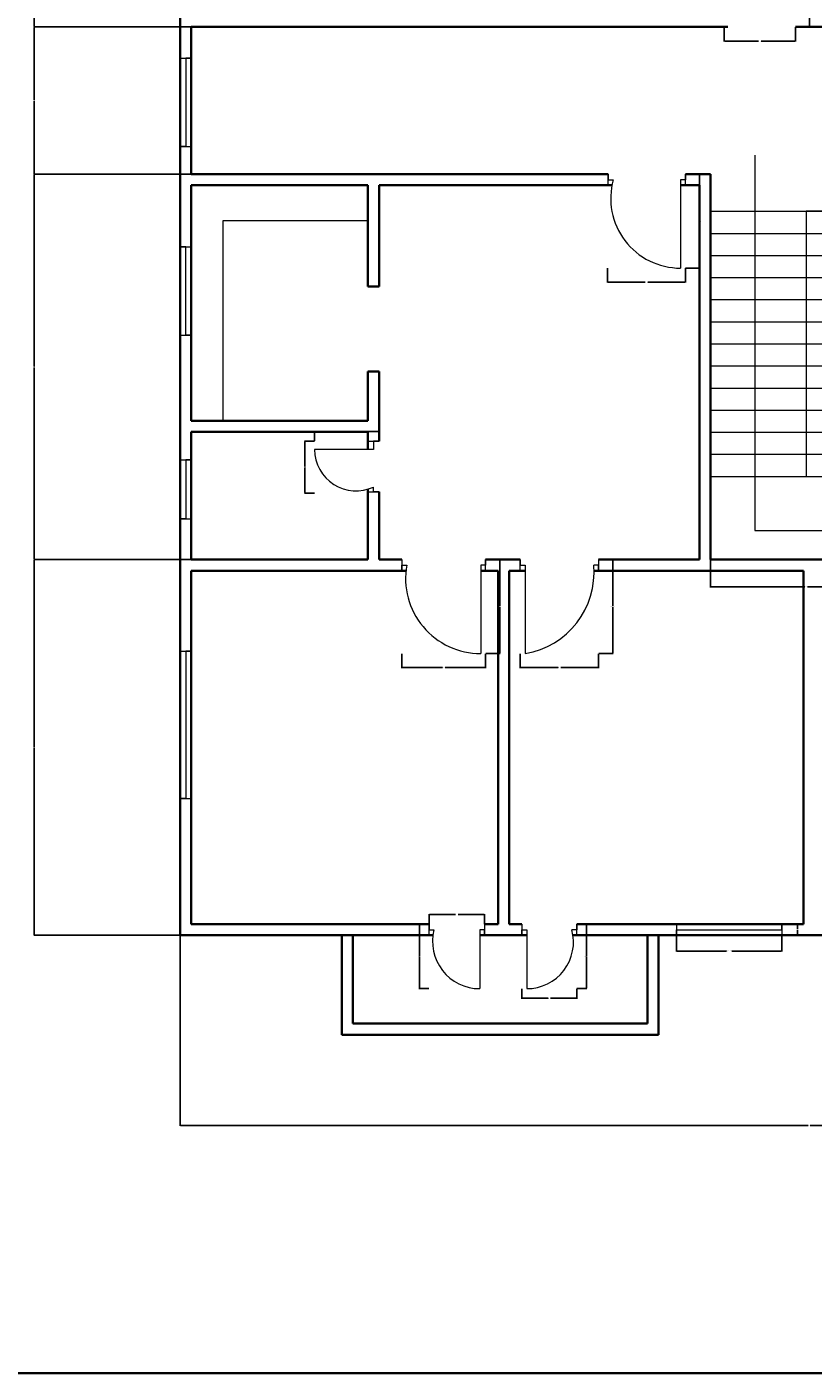
# Model space of a CAD drawing. Units: inches. Extents: x 1944 to 3454, y 1352 to 3055.
# Tile 10 of 17: x 2582 to 2903, y 1352 to 1900. Entities that reach past the tile are written whole.
import ezdxf

# ---------------------------------------------------------------- set-up
doc = ezdxf.new("R2010")
doc.units = ezdxf.units.IN
for name, color, linetype, lineweight in [('A-ANNO-DIMS', 2, 'Continuous', 18), ('A-ANNO-TTLB', 7, 'Continuous', 35), ('A-DOOR', 3, 'Continuous', 20), ('A-FLOR-CASE', 8, 'Continuous', 20), ('A-FLOR-STRS', 7, 'Continuous', 20), ('A-GLAZ', 4, 'Continuous', 18), ('A-WALL', 7, 'Continuous', 35)]:
    doc.layers.add(name, color=color, linetype=linetype, lineweight=lineweight)
doc.styles.get("Standard").update_dxf_attribs({"font": 'arial.ttf'})
doc.dimstyles.get("Standard").update_dxf_attribs({"dimtxt": 0.18, "dimasz": 0.18, "dimexe": 0.18, "dimexo": 0.0625, "dimgap": 0.09, "dimtad": 0, "dimtih": 1, "dimtoh": 1, "dimdec": 4, "dimzin": 0, "dimdsep": 46, "dimtxsty": 'Standard', "dimcen": 0.09, "dimadec": 0, "dimazin": 0, "dimtfac": 1, "dimtdec": 4, "dimtofl": 0, "dimtmove": 0, "dimatfit": 3, "dimfxl": 1, "dimtolj": 1, "dimtzin": 0, "dimarcsym": 0})

# ---------------------------------------------------------------- blocks, each defined once
blk = doc.blocks.new('DOOR-SWING-24IN-08')
for p, q in [((24, 17.34), (0, 17.34)), ((21.75, 20.75), (26.25, 20.75)), ((26.25, 20.75), (24, 20.75)), ((24, 20.75), (24, 19.34)), ((24, 19.34), (24, 17.34)), ((21.75, 0), (26.25, 0)), ((24, 0), (24, 2)), ((26.25, 0), (24, 0))]:
    blk.add_line(p, q)
blk.add_arc((16.9, 17.34), 16.9, 180, 294.8206)
blk = doc.blocks.new('DOOR-SWING-36IN-07')
for p, q in [((0, 38.25), (0, 33.75)), ((0, 33.75), (0, 36)), ((0, 36), (2, 36)), ((34.17, 36), (32.17, 36)), ((32.17, 36), (32.17, 0)), ((34.17, 33.75), (34.17, 38.25)), ((34.17, 38.25), (34.17, 36))]:
    blk.add_line(p, q)
blk.add_arc((32.17, 30.64), 30.64, 169.9223, 270)
blk = doc.blocks.new('DOOR-SWING-36IN-08')
for p, q in [((0, 33.75), (0, 38.25)), ((0, 38.25), (0, 38.25)), ((0, 38.25), (0, 36)), ((0, 36), (2, 36)), ((2, 36), (2, 0)), ((31.9, 36), (29.9, 36)), ((31.9, 38.25), (31.9, 33.75)), ((31.9, 33.75), (31.9, 36))]:
    blk.add_line(p, q)
blk.add_arc((-3.46, 33.05), 33.5, 279.3869, 5.0549)
blk = doc.blocks.new('DOOR-SWING-24IN-09')
for p, q in [((0, 21.75), (0, 26.25)), ((0, 26.25), (0, 24)), ((0, 24), (2, 24)), ((22.65, 24), (20.65, 24)), ((20.65, 24), (20.65, 0)), ((22.65, 26.25), (22.65, 21.75)), ((22.65, 21.75), (22.65, 24)), ((22.65, 21.75), (22.65, 21.75))]:
    blk.add_line(p, q)
blk.add_arc((20.65, 19.25), 19.25, 165.7058, 270)
blk = doc.blocks.new('DOOR-SWING-24IN-10')
for p, q in [((0, 26.25), (0, 21.75)), ((0, 21.75), (0, 24)), ((0, 24), (2, 24)), ((2, 24), (2, 0)), ((22.35, 24), (20.35, 24)), ((22.35, 21.75), (22.35, 26.25)), ((22.35, 26.25), (22.35, 24))]:
    blk.add_line(p, q)
blk.add_arc((2, 19.01), 19.01, 270, 15.2011)
blk = doc.blocks.new('DOOR-SWING-36IN-11')
for p, q in [((0, 33.75), (0, 38.25)), ((0, 38.25), (0, 36)), ((0, 36), (2, 36)), ((31.41, 36), (29.41, 36)), ((29.41, 36), (29.41, 0)), ((31.41, 33.75), (31.41, 38.25)), ((31.41, 38.25), (31.41, 36))]:
    blk.add_line(p, q)
blk.add_arc((29.41, 28.43), 28.43, 164.5673, 270)
blk = doc.blocks.new('WINDOW-PLAN-60.00IN-02')
for p, q in [((2.25, 60), (0, 60)), ((0, 60), (4.5, 60)), ((2.25, 0), (2.25, 60)), ((0, 0), (4.5, 0)), ((4.5, 0), (2.25, 0))]:
    blk.add_line(p, q)
blk = doc.blocks.new('WINDOW-PLAN-36.00IN-01')
for p, q in [((0, 36), (4.5, 36)), ((4.5, 36), (2.25, 36)), ((2.25, 36), (2.25, 0)), ((2.25, 0), (0, 0)), ((0, 0), (4.5, 0))]:
    blk.add_line(p, q)
blk = doc.blocks.new('WINDOW-PLAN-24.00IN-01')
for p, q in [((2.25, 24), (0, 24)), ((0, 24), (4.5, 24)), ((2.25, 0), (2.25, 24)), ((0, 0), (4.5, 0)), ((4.5, 0), (2.25, 0))]:
    blk.add_line(p, q)
blk = doc.blocks.new('WINDOW-PLAN-42.86IN-01')
for p, q in [((0, 4.5), (0, 0)), ((0, 0), (0, 2.25)), ((0, 2.25), (42.86, 2.25)), ((42.86, 2.25), (42.86, 4.5)), ((42.86, 4.5), (42.86, 0))]:
    blk.add_line(p, q)
blk = doc.blocks.new('STAIR-TWO-FLIGHT-01')
for p, q in [((18.12, 152.99), (18.12, 0)), ((0, 130.08), (78, 130.08)), ((78, 130.08), (39, 130.08)), ((39, 130.08), (39, 22.08)), ((0, 121.08), (78, 121.08)), ((0, 112.08), (78, 112.08)), ((0, 103.08), (78, 103.08)), ((0, 94.08), (78, 94.08)), ((0, 85.08), (78, 85.08)), ((0, 76.08), (78, 76.08)), ((0, 67.08), (78, 67.08)), ((61.93, 0), (61.93, 67.08)), ((0, 58.08), (78, 58.08)), ((0, 49.08), (78, 49.08)), ((0, 40.08), (78, 40.08)), ((0, 31.08), (78, 31.08)), ((0, 22.08), (78, 22.08)), ((18.12, 0), (61.93, 0))]:
    blk.add_line(p, q)
blk = doc.blocks.new('*D84')
at = {"layer": 'A-ANNO-DIMS', "color": 0, "lineweight": -2, "transparency": 16777216}
for p, q in [((2847.08, 1530.03), (2847.08, 1523.49)), ((2889.94, 1530.03), (2889.94, 1523.49)), ((2847.26, 1523.67), (2867.39, 1523.67)), ((2889.76, 1523.67), (2869.63, 1523.67))]:
    blk.add_line(p, q, dxfattribs=at)
at = {"layer": 'A-ANNO-DIMS', "color": 0, "transparency": 16777216}
for points in [[(2847.26, 1523.7), (2847.26, 1523.64), (2847.08, 1523.67)], [(2889.76, 1523.7), (2889.76, 1523.64), (2889.94, 1523.67)]]:
    blk.add_solid(points, dxfattribs=at)
at = {"layer": 'Defpoints', "color": 0, "transparency": 16777216}
for p in [(2847.08, 1530.1), (2889.94, 1530.1), (2889.94, 1523.67)]:
    blk.add_point(p, dxfattribs=at)
at = {"layer": 'A-ANNO-DIMS', "color": 0, "transparency": 16777216, "insert": (2868.51, 1523.67), "char_height": 0.18, "attachment_point": 5}
blk.add_mtext('\\A1;WINDOW 43 TYP.', dxfattribs=at)
blk = doc.blocks.new('*D85')
at = {"layer": 'A-ANNO-DIMS', "color": 0, "lineweight": -2, "transparency": 16777216}
for p, q in [((2890, 1534.6), (2896.55, 1534.6)), ((2890, 1530.1), (2896.55, 1530.1)), ((2896.37, 1534.42), (2896.37, 1532.53)), ((2896.37, 1530.28), (2896.37, 1532.16))]:
    blk.add_line(p, q, dxfattribs=at)
at = {"layer": 'A-ANNO-DIMS', "color": 0, "transparency": 16777216}
for points in [[(2896.34, 1534.42), (2896.4, 1534.42), (2896.37, 1534.6)], [(2896.34, 1530.28), (2896.4, 1530.28), (2896.37, 1530.1)]]:
    blk.add_solid(points, dxfattribs=at)
at = {"layer": 'Defpoints', "color": 0, "transparency": 16777216}
for p in [(2889.94, 1534.6), (2889.94, 1530.1), (2896.37, 1534.6)]:
    blk.add_point(p, dxfattribs=at)
at = {"layer": 'A-ANNO-DIMS', "color": 0, "transparency": 16777216, "insert": (2896.37, 1532.35), "char_height": 0.18, "attachment_point": 5}
blk.add_mtext('\\A1;5 TYP.', dxfattribs=at)
blk = doc.blocks.new('*D91')
at = {"layer": 'A-ANNO-DIMS', "color": 0, "lineweight": -2, "transparency": 16777216}
for p, q in [((2860.88, 1694.86), (2860.88, 1671.8)), ((2938.88, 1694.86), (2938.88, 1671.8)), ((2861.06, 1671.98), (2899.35, 1671.98)), ((2938.7, 1671.98), (2900.4, 1671.98))]:
    blk.add_line(p, q, dxfattribs=at)
at = {"layer": 'A-ANNO-DIMS', "color": 0, "transparency": 16777216}
for points in [[(2861.06, 1672.01), (2861.06, 1671.95), (2860.88, 1671.98)], [(2938.7, 1672.01), (2938.7, 1671.95), (2938.88, 1671.98)]]:
    blk.add_solid(points, dxfattribs=at)
at = {"layer": 'Defpoints', "color": 0, "transparency": 16777216}
for p in [(2860.88, 1694.92), (2938.88, 1694.92), (2938.88, 1671.98)]:
    blk.add_point(p, dxfattribs=at)
at = {"layer": 'A-ANNO-DIMS', "color": 0, "transparency": 16777216, "insert": (2899.88, 1671.98), "char_height": 0.18, "attachment_point": 5}
blk.add_mtext('\\A1;78 TYP.', dxfattribs=at)
blk = doc.blocks.new('*D104')
at = {"layer": 'A-ANNO-DIMS', "color": 0, "lineweight": -2, "transparency": 16777216}
for p, q in [((2769.38, 1683.1), (2775.23, 1683.1)), ((2775.05, 1682.92), (2775.05, 1664.15)), ((2775.05, 1645.03), (2775.05, 1663.79)), ((2769.38, 1644.85), (2775.23, 1644.85))]:
    blk.add_line(p, q, dxfattribs=at)
at = {"layer": 'A-ANNO-DIMS', "color": 0, "transparency": 16777216}
for points in [[(2775.02, 1682.92), (2775.08, 1682.92), (2775.05, 1683.1)], [(2775.02, 1645.03), (2775.08, 1645.03), (2775.05, 1644.85)]]:
    blk.add_solid(points, dxfattribs=at)
at = {"layer": 'Defpoints', "color": 0, "transparency": 16777216}
for p in [(2769.32, 1683.1), (2775.05, 1683.1), (2769.32, 1644.85)]:
    blk.add_point(p, dxfattribs=at)
at = {"layer": 'A-ANNO-DIMS', "color": 0, "transparency": 16777216, "insert": (2775.05, 1663.97), "char_height": 0.18, "attachment_point": 5}
blk.add_mtext('\\A1;SWING 38 TYP.', dxfattribs=at)
blk = doc.blocks.new('*D105')
at = {"layer": 'A-ANNO-DIMS', "color": 0, "lineweight": -2, "transparency": 16777216}
for p, q in [((2735.15, 1644.78), (2735.15, 1638.93)), ((2769.32, 1644.78), (2769.32, 1638.93)), ((2735.33, 1639.11), (2751.71, 1639.11)), ((2769.14, 1639.11), (2752.76, 1639.11))]:
    blk.add_line(p, q, dxfattribs=at)
at = {"layer": 'A-ANNO-DIMS', "color": 0, "transparency": 16777216}
for points in [[(2735.33, 1639.14), (2735.33, 1639.08), (2735.15, 1639.11)], [(2769.14, 1639.14), (2769.14, 1639.08), (2769.32, 1639.11)]]:
    blk.add_solid(points, dxfattribs=at)
at = {"layer": 'Defpoints', "color": 0, "transparency": 16777216}
for p in [(2735.15, 1644.85), (2769.32, 1644.85), (2769.32, 1639.11)]:
    blk.add_point(p, dxfattribs=at)
at = {"layer": 'A-ANNO-DIMS', "color": 0, "transparency": 16777216, "insert": (2752.23, 1639.11), "char_height": 0.18, "attachment_point": 5}
blk.add_mtext('\\A1;34 TYP.', dxfattribs=at)
blk = doc.blocks.new('*D106')
at = {"layer": 'A-ANNO-DIMS', "color": 0, "lineweight": -2, "transparency": 16777216}
for p, q in [((2815.41, 1683.1), (2821.26, 1683.1)), ((2821.08, 1682.92), (2821.08, 1664.15)), ((2821.08, 1645.03), (2821.08, 1663.79)), ((2815.41, 1644.85), (2821.26, 1644.85))]:
    blk.add_line(p, q, dxfattribs=at)
at = {"layer": 'A-ANNO-DIMS', "color": 0, "transparency": 16777216}
for points in [[(2821.05, 1682.92), (2821.11, 1682.92), (2821.08, 1683.1)], [(2821.05, 1645.03), (2821.11, 1645.03), (2821.08, 1644.85)]]:
    blk.add_solid(points, dxfattribs=at)
at = {"layer": 'Defpoints', "color": 0, "transparency": 16777216}
for p in [(2815.35, 1683.1), (2821.08, 1683.1), (2815.35, 1644.85)]:
    blk.add_point(p, dxfattribs=at)
at = {"layer": 'A-ANNO-DIMS', "color": 0, "transparency": 16777216, "insert": (2821.08, 1663.97), "char_height": 0.18, "attachment_point": 5}
blk.add_mtext('\\A1;SWING 38 TYP.', dxfattribs=at)
blk = doc.blocks.new('*D107')
at = {"layer": 'A-ANNO-DIMS', "color": 0, "lineweight": -2, "transparency": 16777216}
for p, q in [((2783.44, 1644.78), (2783.44, 1638.93)), ((2815.35, 1644.78), (2815.35, 1638.93)), ((2783.62, 1639.11), (2798.87, 1639.11)), ((2815.17, 1639.11), (2799.92, 1639.11))]:
    blk.add_line(p, q, dxfattribs=at)
at = {"layer": 'A-ANNO-DIMS', "color": 0, "transparency": 16777216}
for points in [[(2783.62, 1639.14), (2783.62, 1639.08), (2783.44, 1639.11)], [(2815.17, 1639.14), (2815.17, 1639.08), (2815.35, 1639.11)]]:
    blk.add_solid(points, dxfattribs=at)
at = {"layer": 'Defpoints', "color": 0, "transparency": 16777216}
for p in [(2783.44, 1644.85), (2815.35, 1644.85), (2815.35, 1639.11)]:
    blk.add_point(p, dxfattribs=at)
at = {"layer": 'A-ANNO-DIMS', "color": 0, "transparency": 16777216, "insert": (2799.39, 1639.11), "char_height": 0.18, "attachment_point": 5}
blk.add_mtext('\\A1;32 TYP.', dxfattribs=at)
blk = doc.blocks.new('*D110')
at = {"layer": 'A-ANNO-DIMS', "color": 0, "lineweight": -2, "transparency": 16777216}
for p, q in [((2895.56, 1938.35), (2901.41, 1938.35)), ((2901.23, 1938.17), (2901.23, 1919.4)), ((2901.23, 1900.28), (2901.23, 1919.04)), ((2895.56, 1900.1), (2901.41, 1900.1))]:
    blk.add_line(p, q, dxfattribs=at)
at = {"layer": 'A-ANNO-DIMS', "color": 0, "transparency": 16777216}
for points in [[(2901.2, 1938.17), (2901.26, 1938.17), (2901.23, 1938.35)], [(2901.2, 1900.28), (2901.26, 1900.28), (2901.23, 1900.1)]]:
    blk.add_solid(points, dxfattribs=at)
at = {"layer": 'Defpoints', "color": 0, "transparency": 16777216}
for p in [(2895.49, 1938.35), (2901.23, 1938.35), (2895.49, 1900.1)]:
    blk.add_point(p, dxfattribs=at)
at = {"layer": 'A-ANNO-DIMS', "color": 0, "transparency": 16777216, "insert": (2901.23, 1919.22), "char_height": 0.18, "attachment_point": 5}
blk.add_mtext('\\A1;SWING 38 TYP.', dxfattribs=at)
blk = doc.blocks.new('*D111')
at = {"layer": 'A-ANNO-DIMS', "color": 0, "lineweight": -2, "transparency": 16777216}
for p, q in [((2866.54, 1900.03), (2866.54, 1894.18)), ((2895.49, 1900.03), (2895.49, 1894.18)), ((2866.72, 1894.36), (2880.49, 1894.36)), ((2895.31, 1894.36), (2881.55, 1894.36))]:
    blk.add_line(p, q, dxfattribs=at)
at = {"layer": 'A-ANNO-DIMS', "color": 0, "transparency": 16777216}
for points in [[(2866.72, 1894.39), (2866.72, 1894.33), (2866.54, 1894.36)], [(2895.31, 1894.39), (2895.31, 1894.33), (2895.49, 1894.36)]]:
    blk.add_solid(points, dxfattribs=at)
at = {"layer": 'Defpoints', "color": 0, "transparency": 16777216}
for p in [(2866.54, 1900.1), (2895.49, 1900.1), (2895.49, 1894.36)]:
    blk.add_point(p, dxfattribs=at)
at = {"layer": 'A-ANNO-DIMS', "color": 0, "transparency": 16777216, "insert": (2881.02, 1894.36), "char_height": 0.18, "attachment_point": 5}
blk.add_mtext('\\A1;29 TYP.', dxfattribs=at)
blk = doc.blocks.new('*D112')
at = {"layer": 'A-ANNO-DIMS', "color": 0, "lineweight": -2, "transparency": 16777216}
for p, q in [((2850.75, 1840.1), (2856.61, 1840.1)), ((2856.43, 1839.92), (2856.43, 1821.15)), ((2856.43, 1802.03), (2856.43, 1820.79)), ((2850.75, 1801.85), (2856.61, 1801.85))]:
    blk.add_line(p, q, dxfattribs=at)
at = {"layer": 'A-ANNO-DIMS', "color": 0, "transparency": 16777216}
for points in [[(2856.4, 1839.92), (2856.46, 1839.92), (2856.43, 1840.1)], [(2856.4, 1802.03), (2856.46, 1802.03), (2856.43, 1801.85)]]:
    blk.add_solid(points, dxfattribs=at)
at = {"layer": 'Defpoints', "color": 0, "transparency": 16777216}
for p in [(2850.69, 1840.1), (2856.43, 1840.1), (2850.69, 1801.85)]:
    blk.add_point(p, dxfattribs=at)
at = {"layer": 'A-ANNO-DIMS', "color": 0, "transparency": 16777216, "insert": (2856.43, 1820.97), "char_height": 0.18, "attachment_point": 5}
blk.add_mtext('\\A1;SWING 38 TYP.', dxfattribs=at)
blk = doc.blocks.new('*D113')
at = {"layer": 'A-ANNO-DIMS', "color": 0, "lineweight": -2, "transparency": 16777216}
for p, q in [((2818.92, 1801.78), (2818.92, 1795.93)), ((2850.69, 1801.78), (2850.69, 1795.93)), ((2819.1, 1796.11), (2834.27, 1796.11)), ((2850.51, 1796.11), (2835.33, 1796.11))]:
    blk.add_line(p, q, dxfattribs=at)
at = {"layer": 'A-ANNO-DIMS', "color": 0, "transparency": 16777216}
for points in [[(2819.1, 1796.14), (2819.1, 1796.08), (2818.92, 1796.11)], [(2850.51, 1796.14), (2850.51, 1796.08), (2850.69, 1796.11)]]:
    blk.add_solid(points, dxfattribs=at)
at = {"layer": 'Defpoints', "color": 0, "transparency": 16777216}
for p in [(2818.92, 1801.85), (2850.69, 1801.85), (2850.69, 1796.11)]:
    blk.add_point(p, dxfattribs=at)
at = {"layer": 'A-ANNO-DIMS', "color": 0, "transparency": 16777216, "insert": (2834.8, 1796.11), "char_height": 0.18, "attachment_point": 5}
blk.add_mtext('\\A1;32 TYP.', dxfattribs=at)
blk = doc.blocks.new('*D130')
at = {"layer": 'A-ANNO-DIMS', "color": 0, "lineweight": -2, "transparency": 16777216}
for p, q in [((2699.63, 1731.48), (2699.63, 1735.53)), ((2699.81, 1735.35), (2711.76, 1735.35)), ((2725.7, 1735.35), (2713.74, 1735.35)), ((2725.88, 1731.48), (2725.88, 1735.53))]:
    blk.add_line(p, q, dxfattribs=at)
at = {"layer": 'A-ANNO-DIMS', "color": 0, "transparency": 16777216}
for points in [[(2699.81, 1735.38), (2699.81, 1735.32), (2699.63, 1735.35)], [(2725.7, 1735.38), (2725.7, 1735.32), (2725.88, 1735.35)]]:
    blk.add_solid(points, dxfattribs=at)
at = {"layer": 'Defpoints', "color": 0, "transparency": 16777216}
for p in [(2725.88, 1735.35), (2699.63, 1731.41), (2725.88, 1731.41)]:
    blk.add_point(p, dxfattribs=at)
at = {"layer": 'A-ANNO-DIMS', "color": 0, "transparency": 16777216, "insert": (2712.75, 1735.35), "char_height": 0.18, "attachment_point": 5}
blk.add_mtext('\\A1;SWING 26 TYP.', dxfattribs=at)
blk = doc.blocks.new('*D131')
at = {"layer": 'A-ANNO-DIMS', "color": 0, "lineweight": -2, "transparency": 16777216}
for p, q in [((2699.56, 1731.41), (2695.51, 1731.41)), ((2695.69, 1731.23), (2695.69, 1721.01)), ((2695.69, 1710.42), (2695.69, 1720.65)), ((2699.56, 1710.24), (2695.51, 1710.24))]:
    blk.add_line(p, q, dxfattribs=at)
at = {"layer": 'A-ANNO-DIMS', "color": 0, "transparency": 16777216}
for points in [[(2695.66, 1731.23), (2695.72, 1731.23), (2695.69, 1731.41)], [(2695.66, 1710.42), (2695.72, 1710.42), (2695.69, 1710.24)]]:
    blk.add_solid(points, dxfattribs=at)
at = {"layer": 'Defpoints', "color": 0, "transparency": 16777216}
for p in [(2695.69, 1731.41), (2699.63, 1731.41), (2699.63, 1710.24)]:
    blk.add_point(p, dxfattribs=at)
at = {"layer": 'A-ANNO-DIMS', "color": 0, "transparency": 16777216, "insert": (2695.69, 1720.83), "char_height": 0.18, "attachment_point": 5}
blk.add_mtext('\\A1;21 TYP.', dxfattribs=at)
blk = doc.blocks.new('*D132')
at = {"layer": 'A-ANNO-DIMS', "color": 0, "lineweight": -2, "transparency": 16777216}
for p, q in [((2746.19, 1534.6), (2742.14, 1534.6)), ((2742.32, 1534.42), (2742.32, 1521.65)), ((2742.32, 1508.53), (2742.32, 1521.29)), ((2746.19, 1508.35), (2742.14, 1508.35))]:
    blk.add_line(p, q, dxfattribs=at)
at = {"layer": 'A-ANNO-DIMS', "color": 0, "transparency": 16777216}
for points in [[(2742.29, 1534.42), (2742.35, 1534.42), (2742.32, 1534.6)], [(2742.29, 1508.53), (2742.35, 1508.53), (2742.32, 1508.35)]]:
    blk.add_solid(points, dxfattribs=at)
at = {"layer": 'Defpoints', "color": 0, "transparency": 16777216}
for p in [(2742.32, 1534.6), (2746.26, 1534.6), (2746.26, 1508.35)]:
    blk.add_point(p, dxfattribs=at)
at = {"layer": 'A-ANNO-DIMS', "color": 0, "transparency": 16777216, "insert": (2742.32, 1521.47), "char_height": 0.18, "attachment_point": 5}
blk.add_mtext('\\A1;SWING 26 TYP.', dxfattribs=at)
blk = doc.blocks.new('*D133')
at = {"layer": 'A-ANNO-DIMS', "color": 0, "lineweight": -2, "transparency": 16777216}
for p, q in [((2746.26, 1534.66), (2746.26, 1538.71)), ((2746.44, 1538.53), (2757.05, 1538.53)), ((2768.73, 1538.53), (2758.11, 1538.53)), ((2768.91, 1534.66), (2768.91, 1538.71))]:
    blk.add_line(p, q, dxfattribs=at)
at = {"layer": 'A-ANNO-DIMS', "color": 0, "transparency": 16777216}
for points in [[(2746.44, 1538.56), (2746.44, 1538.5), (2746.26, 1538.53)], [(2768.73, 1538.56), (2768.73, 1538.5), (2768.91, 1538.53)]]:
    blk.add_solid(points, dxfattribs=at)
at = {"layer": 'Defpoints', "color": 0, "transparency": 16777216}
for p in [(2768.91, 1538.53), (2746.26, 1534.6), (2768.91, 1534.6)]:
    blk.add_point(p, dxfattribs=at)
at = {"layer": 'A-ANNO-DIMS', "color": 0, "transparency": 16777216, "insert": (2757.58, 1538.53), "char_height": 0.18, "attachment_point": 5}
blk.add_mtext('\\A1;23 TYP.', dxfattribs=at)
blk = doc.blocks.new('*D134')
at = {"layer": 'A-ANNO-DIMS', "color": 0, "lineweight": -2, "transparency": 16777216}
for p, q in [((2806.5, 1534.6), (2810.56, 1534.6)), ((2810.38, 1534.42), (2810.38, 1521.65)), ((2810.38, 1508.53), (2810.38, 1521.29)), ((2806.5, 1508.35), (2810.56, 1508.35))]:
    blk.add_line(p, q, dxfattribs=at)
at = {"layer": 'A-ANNO-DIMS', "color": 0, "transparency": 16777216}
for points in [[(2810.35, 1534.42), (2810.41, 1534.42), (2810.38, 1534.6)], [(2810.35, 1508.53), (2810.41, 1508.53), (2810.38, 1508.35)]]:
    blk.add_solid(points, dxfattribs=at)
at = {"layer": 'Defpoints', "color": 0, "transparency": 16777216}
for p in [(2806.44, 1534.6), (2810.38, 1534.6), (2806.44, 1508.35)]:
    blk.add_point(p, dxfattribs=at)
at = {"layer": 'A-ANNO-DIMS', "color": 0, "transparency": 16777216, "insert": (2810.38, 1521.47), "char_height": 0.18, "attachment_point": 5}
blk.add_mtext('\\A1;SWING 26 TYP.', dxfattribs=at)
blk = doc.blocks.new('*D135')
at = {"layer": 'A-ANNO-DIMS', "color": 0, "lineweight": -2, "transparency": 16777216}
for p, q in [((2784.09, 1508.28), (2784.09, 1504.23)), ((2806.44, 1508.28), (2806.44, 1504.23)), ((2784.27, 1504.41), (2794.74, 1504.41)), ((2806.26, 1504.41), (2795.8, 1504.41))]:
    blk.add_line(p, q, dxfattribs=at)
at = {"layer": 'A-ANNO-DIMS', "color": 0, "transparency": 16777216}
for points in [[(2784.27, 1504.44), (2784.27, 1504.38), (2784.09, 1504.41)], [(2806.26, 1504.44), (2806.26, 1504.38), (2806.44, 1504.41)]]:
    blk.add_solid(points, dxfattribs=at)
at = {"layer": 'Defpoints', "color": 0, "transparency": 16777216}
for p in [(2784.09, 1508.35), (2806.44, 1508.35), (2806.44, 1504.41)]:
    blk.add_point(p, dxfattribs=at)
at = {"layer": 'A-ANNO-DIMS', "color": 0, "transparency": 16777216, "insert": (2795.27, 1504.41), "char_height": 0.18, "attachment_point": 5}
blk.add_mtext('\\A1;22 TYP.', dxfattribs=at)
blk = doc.blocks.new('*D186')
at = {"layer": 'A-ANNO-DIMS', "color": 0, "lineweight": -2, "transparency": 16777216}
for p, q in [((2644.88, 1530.03), (2644.88, 1452.42)), ((3157.38, 1530.03), (3157.38, 1452.42)), ((2645.06, 1452.6), (2900.73, 1452.6)), ((3157.2, 1452.6), (2901.52, 1452.6))]:
    blk.add_line(p, q, dxfattribs=at)
at = {"layer": 'A-ANNO-DIMS', "color": 0, "transparency": 16777216}
for points in [[(2645.06, 1452.63), (2645.06, 1452.57), (2644.88, 1452.6)], [(3157.2, 1452.63), (3157.2, 1452.57), (3157.38, 1452.6)]]:
    blk.add_solid(points, dxfattribs=at)
at = {"layer": 'Defpoints', "color": 0, "transparency": 16777216}
for p in [(2644.88, 1530.1), (3157.38, 1530.1), (3157.38, 1452.6)]:
    blk.add_point(p, dxfattribs=at)
at = {"layer": 'A-ANNO-DIMS', "color": 0, "transparency": 16777216, "insert": (2901.13, 1452.6), "char_height": 0.18, "attachment_point": 5}
blk.add_mtext('\\A1;512.5', dxfattribs=at)
blk = doc.blocks.new('*D189')
at = {"layer": 'A-ANNO-DIMS', "color": 0, "lineweight": -2, "transparency": 16777216}
for p, q in [((2649.31, 2033.6), (2585.24, 2033.6)), ((2585.42, 2033.42), (2585.42, 1967.03)), ((2585.42, 1900.28), (2585.42, 1966.66)), ((2649.31, 1900.1), (2585.24, 1900.1))]:
    blk.add_line(p, q, dxfattribs=at)
at = {"layer": 'A-ANNO-DIMS', "color": 0, "transparency": 16777216}
for points in [[(2585.39, 2033.42), (2585.45, 2033.42), (2585.42, 2033.6)], [(2585.39, 1900.28), (2585.45, 1900.28), (2585.42, 1900.1)]]:
    blk.add_solid(points, dxfattribs=at)
at = {"layer": 'Defpoints', "color": 0, "transparency": 16777216}
for p in [(2649.38, 2033.6), (2585.42, 1900.1), (2649.38, 1900.1)]:
    blk.add_point(p, dxfattribs=at)
at = {"layer": 'A-ANNO-DIMS', "color": 0, "transparency": 16777216, "insert": (2585.42, 1966.85), "char_height": 0.18, "attachment_point": 5}
blk.add_mtext('\\A1;133.5', dxfattribs=at)
blk = doc.blocks.new('*D190')
at = {"layer": 'A-ANNO-DIMS', "color": 0, "lineweight": -2, "transparency": 16777216}
for p, q in [((2649.31, 1900.1), (2585.24, 1900.1)), ((2585.42, 1899.92), (2585.42, 1870.28)), ((2585.42, 1840.28), (2585.42, 1869.91)), ((2649.31, 1840.1), (2585.24, 1840.1))]:
    blk.add_line(p, q, dxfattribs=at)
at = {"layer": 'A-ANNO-DIMS', "color": 0, "transparency": 16777216}
for points in [[(2585.39, 1899.92), (2585.45, 1899.92), (2585.42, 1900.1)], [(2585.39, 1840.28), (2585.45, 1840.28), (2585.42, 1840.1)]]:
    blk.add_solid(points, dxfattribs=at)
at = {"layer": 'Defpoints', "color": 0, "transparency": 16777216}
for p in [(2649.38, 1900.1), (2585.42, 1840.1), (2649.38, 1840.1)]:
    blk.add_point(p, dxfattribs=at)
at = {"layer": 'A-ANNO-DIMS', "color": 0, "transparency": 16777216, "insert": (2585.42, 1870.1), "char_height": 0.18, "attachment_point": 5}
blk.add_mtext('\\A1;60', dxfattribs=at)
blk = doc.blocks.new('*D191')
at = {"layer": 'A-ANNO-DIMS', "color": 0, "lineweight": -2, "transparency": 16777216}
for p, q in [((2649.31, 1840.1), (2585.24, 1840.1)), ((2585.42, 1839.92), (2585.42, 1761.78)), ((2585.42, 1683.28), (2585.42, 1761.41)), ((2649.31, 1683.1), (2585.24, 1683.1))]:
    blk.add_line(p, q, dxfattribs=at)
at = {"layer": 'A-ANNO-DIMS', "color": 0, "transparency": 16777216}
for points in [[(2585.39, 1839.92), (2585.45, 1839.92), (2585.42, 1840.1)], [(2585.39, 1683.28), (2585.45, 1683.28), (2585.42, 1683.1)]]:
    blk.add_solid(points, dxfattribs=at)
at = {"layer": 'Defpoints', "color": 0, "transparency": 16777216}
for p in [(2649.38, 1840.1), (2585.42, 1683.1), (2649.38, 1683.1)]:
    blk.add_point(p, dxfattribs=at)
at = {"layer": 'A-ANNO-DIMS', "color": 0, "transparency": 16777216, "insert": (2585.42, 1761.6), "char_height": 0.18, "attachment_point": 5}
blk.add_mtext('\\A1;157', dxfattribs=at)
blk = doc.blocks.new('*D192')
at = {"layer": 'A-ANNO-DIMS', "color": 0, "lineweight": -2, "transparency": 16777216}
for p, q in [((2649.31, 1683.1), (2585.24, 1683.1)), ((2585.42, 1682.92), (2585.42, 1606.78)), ((2585.42, 1530.28), (2585.42, 1606.41)), ((2644.81, 1530.1), (2585.24, 1530.1))]:
    blk.add_line(p, q, dxfattribs=at)
at = {"layer": 'A-ANNO-DIMS', "color": 0, "transparency": 16777216}
for points in [[(2585.39, 1682.92), (2585.45, 1682.92), (2585.42, 1683.1)], [(2585.39, 1530.28), (2585.45, 1530.28), (2585.42, 1530.1)]]:
    blk.add_solid(points, dxfattribs=at)
at = {"layer": 'Defpoints', "color": 0, "transparency": 16777216}
for p in [(2649.38, 1683.1), (2585.42, 1530.1), (2644.88, 1530.1)]:
    blk.add_point(p, dxfattribs=at)
at = {"layer": 'A-ANNO-DIMS', "color": 0, "transparency": 16777216, "insert": (2585.42, 1606.6), "char_height": 0.18, "attachment_point": 5}
blk.add_mtext('\\A1;153', dxfattribs=at)

msp = doc.modelspace()

# ---------------------------------------------------------------- linework, layer by layer
at = {"layer": 'A-ANNO-TTLB'}
msp.add_lwpolyline([(1943.914, 3054.605), (3453.633, 3054.605), (3453.633, 1351.76), (1943.914, 1351.76)], close=True, dxfattribs=at)
at = {"layer": 'A-FLOR-CASE'}
for p, q in [((2721.375, 1821.056), (2662.255, 1821.056)), ((2662.255, 1821.056), (2662.255, 1739.596))]:
    msp.add_line(p, q, dxfattribs=at)
at = {"layer": 'A-WALL'}
for p, q in [((2644.875, 2182.096), (2644.875, 1530.096)), ((2649.375, 1900.096), (2649.375, 1840.096)), ((2737.875, 1900.096), (2649.375, 1900.096)), ((2649.375, 1900.096), (2649.375, 1840.096)), ((2737.875, 1900.096), (2868.046, 1900.096)), ((2895.494, 1900.096), (2906.831, 1900.096)), ((2649.375, 1840.096), (2819.28, 1840.096)), ((2850.688, 1840.096), (2860.875, 1840.096)), ((2860.875, 1840.096), (2860.875, 1683.096)), ((2649.375, 1835.596), (2649.375, 1739.596)), ((2649.375, 1835.596), (2721.375, 1835.596)), ((2721.375, 1835.596), (2721.375, 1794.415)), ((2725.875, 1835.596), (2725.875, 1794.415)), ((2725.875, 1835.596), (2820.756, 1835.596)), ((2848.688, 1835.596), (2856.375, 1835.596)), ((2856.375, 1683.096), (2856.375, 1835.596)), ((2721.375, 1794.415), (2725.875, 1794.415)), ((2721.375, 1759.737), (2721.375, 1739.596)), ((2721.375, 1759.737), (2725.875, 1759.737)), ((2725.875, 1759.737), (2725.875, 1731.415)), ((2649.375, 1739.596), (2721.375, 1739.596)), ((2649.375, 1735.096), (2649.375, 1683.096)), ((2649.375, 1735.096), (2721.375, 1735.096)), ((2721.375, 1735.096), (2721.375, 1728.003)), ((2721.375, 1711.808), (2721.375, 1683.096)), ((2725.875, 1710.66), (2725.875, 1683.096)), ((2649.375, 1683.096), (2721.375, 1683.096)), ((2649.375, 1678.596), (2649.375, 1534.596)), ((2649.375, 1678.596), (2736.837, 1678.596)), ((2725.875, 1683.096), (2735.151, 1683.096)), ((2767.317, 1678.596), (2774.375, 1678.596)), ((2769.317, 1683.096), (2783.443, 1683.096)), ((2774.375, 1678.596), (2774.375, 1534.596)), ((2778.875, 1678.596), (2778.875, 1534.596)), ((2778.875, 1678.596), (2785.443, 1678.596)), ((2813.469, 1678.596), (2898.875, 1678.596)), ((2815.346, 1683.096), (2856.375, 1683.096)), ((2860.875, 1683.096), (2938.875, 1683.096)), ((2898.875, 1678.596), (2898.875, 1534.596)), ((2644.875, 1530.096), (2747.824, 1530.096)), ((2649.375, 1534.596), (2746.256, 1534.596)), ((2710.727, 1489.596), (2710.727, 1530.096)), ((2715.227, 1530.096), (2715.227, 1494.096)), ((2766.908, 1530.096), (2786.093, 1530.096)), ((2768.908, 1534.596), (2774.375, 1534.596)), ((2778.875, 1534.596), (2784.093, 1534.596)), ((2804.91, 1530.096), (2998.902, 1530.096)), ((2806.442, 1534.596), (2898.875, 1534.596)), ((2835.227, 1494.096), (2835.227, 1530.096)), ((2839.727, 1530.096), (2839.727, 1494.096)), ((2715.227, 1494.096), (2835.227, 1494.096)), ((2839.727, 1494.096), (2839.727, 1489.596)), ((2715.227, 1489.596), (2710.727, 1489.596)), ((2839.727, 1489.596), (2715.227, 1489.596))]:
    msp.add_line(p, q, dxfattribs=at)

# ---------------------------------------------------------------- block references
at = {"layer": 'A-DOOR'}
for name, p in [('DOOR-SWING-36IN-11', (2819.28, 1801.846)), ('DOOR-SWING-24IN-08', (2699.626, 1710.66)), ('DOOR-SWING-36IN-07', (2735.151, 1644.846)), ('DOOR-SWING-36IN-08', (2783.443, 1644.846)), ('DOOR-SWING-24IN-09', (2746.257, 1508.346)), ('DOOR-SWING-24IN-10', (2784.094, 1508.346))]:
    msp.add_blockref(name, p, dxfattribs=at)
at = {"layer": 'A-FLOR-STRS'}
msp.add_blockref('STAIR-TWO-FLIGHT-01', (2860.876, 1694.924), dxfattribs=at)
at = {"layer": 'A-GLAZ'}
for name, p in [('WINDOW-PLAN-36.00IN-01', (2644.876, 1851.362)), ('WINDOW-PLAN-42.86IN-01', (2847.083, 1530.096))]:
    msp.add_blockref(name, p, dxfattribs=at)
at = {"layer": 'A-GLAZ', "extrusion": (0, 0, -1), "zscale": -1, "rotation": 180}
for name, p in [('WINDOW-PLAN-36.00IN-01', (-2644.876, 1810.528)), ('WINDOW-PLAN-24.00IN-01', (-2644.876, 1723.746)), ('WINDOW-PLAN-60.00IN-02', (-2644.876, 1645.752))]:
    msp.add_blockref(name, p, dxfattribs=at)

# ---------------------------------------------------------------- dimensions: what is measured, and where the dimension line sits
at = {"layer": 'A-ANNO-DIMS'}
for base, p1, p2, override, picture, middle in [((2585.416, 1900.096), (2649.375, 2033.596), (2649.375, 1900.096), {"dimdec": 1, "dimlfac": 1, "dimrnd": 0, "dimzin": 0, "dimdsep": 46, "dimlunit": 2}, '*D189', (2585.416, 1966.846)), ((2585.416, 1840.096), (2649.375, 1900.096), (2649.375, 1840.096), {"dimdec": 0, "dimlfac": 1, "dimrnd": 0, "dimzin": 0, "dimdsep": 46, "dimlunit": 2}, '*D190', (2585.416, 1870.096)), ((2585.416, 1683.096), (2649.375, 1840.096), (2649.375, 1683.096), {"dimdec": 0, "dimlfac": 1, "dimrnd": 0, "dimzin": 0, "dimdsep": 46, "dimlunit": 2}, '*D191', (2585.416, 1761.596)), ((2585.416, 1530.096), (2649.375, 1683.096), (2644.875, 1530.096), {"dimdec": 0, "dimlfac": 1, "dimrnd": 0, "dimzin": 0, "dimdsep": 46, "dimlunit": 2}, '*D192', (2585.416, 1606.596))]:
    dim = msp.add_linear_dim(base=base, p1=p1, p2=p2, angle=90, dimstyle='Standard', override=override, dxfattribs=at)
    dim.commit()
    dim.dimension.update_dxf_attribs({"geometry": picture, "text_midpoint": middle})
for base, p1, p2, text, picture, middle in [((2901.232, 1938.346), (2895.494, 1900.096), (2895.494, 1938.346), 'SWING <> TYP.', '*D110', (2901.232, 1919.221)), ((2856.426, 1840.096), (2850.688, 1801.846), (2850.688, 1840.096), 'SWING <> TYP.', '*D112', (2856.426, 1820.971)), ((2695.688, 1731.415), (2699.625, 1710.239), (2699.625, 1731.415), '<> TYP.', '*D131', (2695.688, 1720.827)), ((2775.054, 1683.096), (2769.317, 1644.846), (2769.317, 1683.096), 'SWING <> TYP.', '*D104', (2775.054, 1663.971)), ((2821.084, 1683.096), (2815.346, 1644.846), (2815.346, 1683.096), 'SWING <> TYP.', '*D106', (2821.084, 1663.971)), ((2742.319, 1534.596), (2746.256, 1508.346), (2746.256, 1534.596), 'SWING <> TYP.', '*D132', (2742.319, 1521.471)), ((2810.38, 1534.596), (2806.442, 1508.346), (2806.442, 1534.596), 'SWING <> TYP.', '*D134', (2810.38, 1521.471)), ((2896.366221709, 1534.596365033), (2889.937993744, 1530.096365033), (2889.937993744, 1534.596365033), '<> TYP.', '*D85', (2896.366221709, 1532.346365033))]:
    dim = msp.add_linear_dim(base=base, p1=p1, p2=p2, angle=90, text=text, dimstyle='Standard', override={"dimdec": 0, "dimlfac": 1, "dimrnd": 0, "dimzin": 0, "dimdsep": 46, "dimlunit": 2}, dxfattribs=at)
    dim.commit()
    dim.dimension.update_dxf_attribs({"geometry": picture, "text_midpoint": middle})
for base, p1, p2, text, picture, middle in [((2895.494, 1894.359), (2866.541, 1900.096), (2895.494, 1900.096), '<> TYP.', '*D111', (2881.018, 1894.359)), ((2850.688, 1796.109), (2818.917, 1801.846), (2850.688, 1801.846), '<> TYP.', '*D113', (2834.803, 1796.109)), ((2725.875, 1735.352), (2699.625, 1731.415), (2725.875, 1731.415), 'SWING <> TYP.', '*D130', (2712.75, 1735.352)), ((2938.875, 1671.976), (2860.875, 1694.924), (2938.875, 1694.924), '<> TYP.', '*D91', (2899.875, 1671.976)), ((2769.317, 1639.109), (2735.151, 1644.846), (2769.317, 1644.846), '<> TYP.', '*D105', (2752.234, 1639.109)), ((2815.346, 1639.109), (2783.443, 1644.846), (2815.346, 1644.846), '<> TYP.', '*D107', (2799.395, 1639.109)), ((2768.908, 1538.534), (2746.256, 1534.596), (2768.908, 1534.596), '<> TYP.', '*D133', (2757.582, 1538.534)), ((2889.938, 1523.668), (2847.083, 1530.096), (2889.938, 1530.096), 'WINDOW <> TYP.', '*D84', (2868.511, 1523.668)), ((2806.442, 1504.409), (2784.093, 1508.346), (2806.442, 1508.346), '<> TYP.', '*D135', (2795.268, 1504.409))]:
    dim = msp.add_linear_dim(base=base, p1=p1, p2=p2, text=text, dimstyle='Standard', override={"dimdec": 0, "dimlfac": 1, "dimrnd": 0, "dimzin": 0, "dimdsep": 46, "dimlunit": 2}, dxfattribs=at)
    dim.commit()
    dim.dimension.update_dxf_attribs({"geometry": picture, "text_midpoint": middle})
dim = msp.add_linear_dim(base=(3157.375, 1452.596), p1=(2644.875, 1530.096), p2=(3157.375, 1530.096), dimstyle='Standard', override={"dimdec": 1, "dimlfac": 1, "dimrnd": 0, "dimzin": 0, "dimdsep": 46, "dimlunit": 2}, dxfattribs=at)
dim.commit()
dim.dimension.update_dxf_attribs({"geometry": '*D186', "text_midpoint": (2901.125, 1452.596)})

doc.saveas('drawing.dxf')
